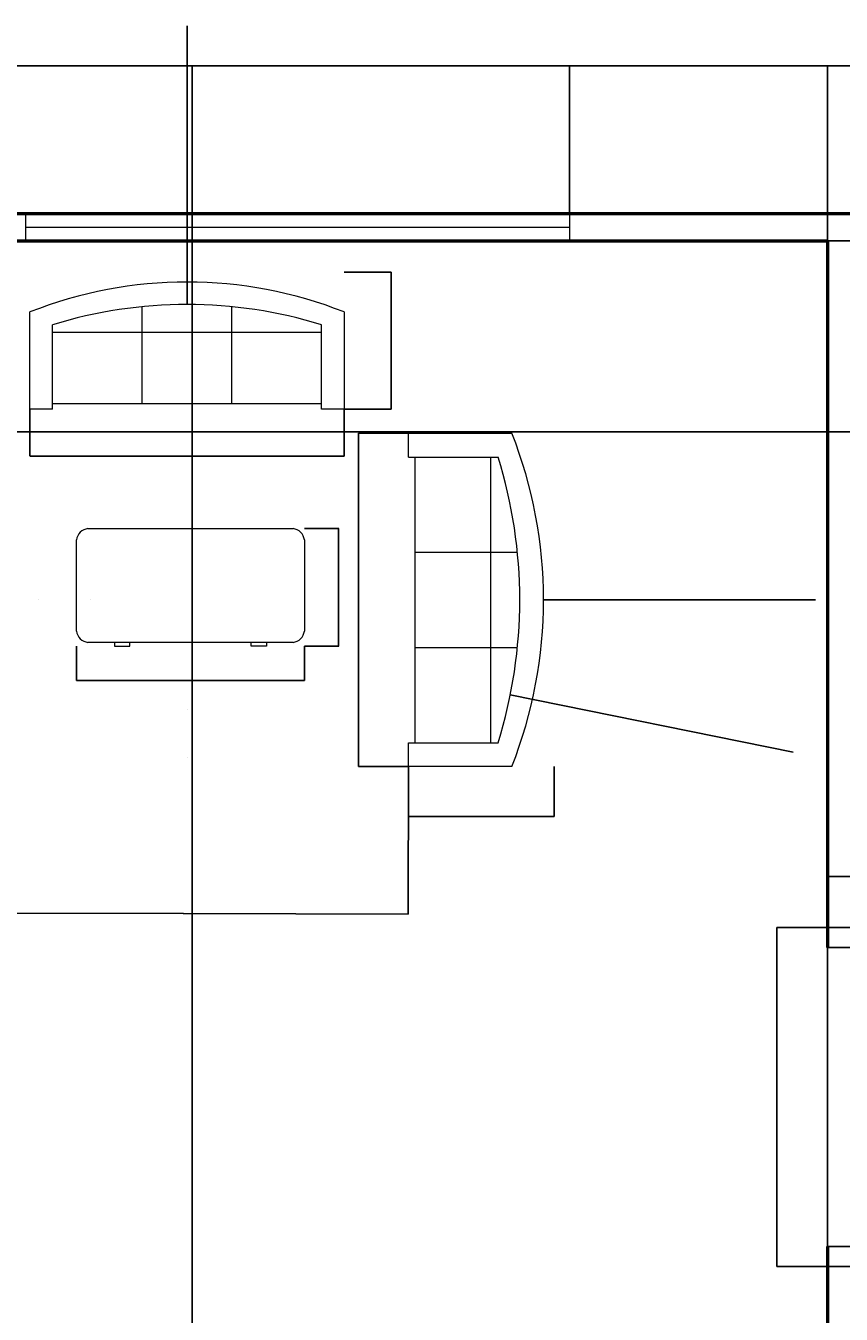
# Model space of a CAD drawing. Units: millimetres. Extents: x 1584 to 12772, y -932 to 10602.
# Tile 4 of 4: x 6178 to 9178, y 5860 to 10602. Entities that reach past the tile are written whole.
import ezdxf

# ---------------------------------------------------------------- set-up
doc = ezdxf.new("R2010")
doc.units = ezdxf.units.MM
for name, color, linetype, lineweight in [('A-ANNO-DIMS', 2, 'Continuous', 18), ('A-DOOR', 3, 'Continuous', 25), ('A-FURN', 8, 'Continuous', 18), ('A-GLAZ', 4, 'Continuous', 18), ('A-WALL', 7, 'Continuous', 50)]:
    doc.layers.add(name, color=color, linetype=linetype, lineweight=lineweight)
doc.styles.get("Standard").update_dxf_attribs({"font": 'arial.ttf'})
doc.dimstyles.get("Standard").update_dxf_attribs({"dimtxt": 0.18, "dimasz": 0.18, "dimexe": 0.18, "dimexo": 0.0625, "dimgap": 0.09, "dimtad": 0, "dimtih": 1, "dimtoh": 1, "dimdec": 4, "dimzin": 0, "dimdsep": 46, "dimtxsty": 'Standard', "dimcen": 0.09, "dimadec": 0, "dimazin": 0, "dimtfac": 1, "dimtdec": 4, "dimtofl": 0, "dimtmove": 0, "dimatfit": 3, "dimfxl": 1, "dimtolj": 1, "dimtzin": 0, "dimarcsym": 0})

# ---------------------------------------------------------------- blocks, each defined once
blk = doc.blocks.new('Sofa - Roundback 7 ft.')
for p, q in [((-12.00002, -32.44210000000393), (-12.00003, -6.597100000003898)), ((11.99996999999999, -32.44210000000393), (11.99997999999999, -6.597100000003898)), ((-36.000027, -34.00000000000395), (-36.000027, -11.46960000000396)), ((35.99997999999999, -34.00000000000395), (35.99997999999999, -11.46960000000396)), ((-35.999844, -13.38190000000397), (35.99979999999999, -13.38190000000397)), ((-36.000027, -32.44210000000393), (35.99997999999999, -32.44210000000393))]:
    blk.add_line(p, q)
for points in [[(-36.000027, -34.00000000000395), (-42.000027, -34.00000000000395), (-42.000027, -8.000000000003944)], [(41.99997999999999, -8.000000000003944), (41.99997999999999, -34.00000000000395), (35.99997999999999, -34.00000000000395)]]:
    blk.add_lwpolyline(points)
for centre, radius, start, end in [((0, -114.2500000000039), 114.2500000000039, 68.43141000000072, 111.5686000000006), ((-1.00000000032e-05, -127.1968000000039), 121.1967999999973, 72.72032999999948, 107.2797000000005)]:
    blk.add_arc(centre, radius, start, end)
blk = doc.blocks.new('Desk - 30 x 60 in.')
for p, q in [((-26.999995, 0), (26.999995, 0)), ((-29.999995, -27), (-29.999995, -3)), ((29.999995, -3), (29.999995, -27)), ((26.999995, -30), (-26.999995, -30)), ((-20.000005, -30), (-20.000005, -31)), ((-16.000005, -31), (-16.000005, -30)), ((15.999995, -31), (15.999995, -30)), ((19.999995, -30), (19.999995, -31)), ((-20.000005, -31), (-16.000005, -31)), ((19.999995, -31), (15.999995, -31))]:
    blk.add_line(p, q)
for centre, radius, start, end in [((-26.499995, -3.5), 3.535534000004229, 98.1300999999916, 171.8698999999352), ((26.499995, -3.5), 3.535533999997753, 8.130102000022115, 81.8698999999439), ((-26.499995, -26.5), 3.535534000000845, 188.1301000000653, 261.8699000000085), ((26.499995, -26.5), 3.535534000004826, 278.1301000000561, 351.8698999999439)]:
    blk.add_arc(centre, radius, start, end)
blk = doc.blocks.new('DOOR-SINGLE-1000')
for p, q in [((1000.000230036349, 1174.20008536707), (1000.000230036349, 1248.400085367071)), ((1000.000230036349, 1248.400085367071), (1100.000230036349, 1248.400085367071)), ((1100.000230036349, 1248.400085367071), (1100.000230036349, 1174.20008536707)), ((1000.000230036349, 1174.20008536707), (0.0002300363494214, 1174.20008536707)), ((0.0002300363494214, 1174.20008536707), (0.0002300363494214, 1074.200085367071)), ((1000.000230036349, 1074.200085367071), (1000.000230036349, 1174.20008536707)), ((1100.000230036349, 1174.20008536707), (1000.000230036349, 1174.20008536707)), ((0.0002300363494214, 1074.200085367071), (1000.000230036349, 1074.200085367071)), ((1000.000230036349, 8.53670690049e-05), (1000.000230036349, 74.20008536706973)), ((1000.000230036349, 74.20008536706973), (1100.000230036349, 74.20008536706973)), ((1100.000230036349, 74.20008536706973), (1100.000230036349, 8.53670690049e-05)), ((1100.000230036349, 8.53670690049e-05), (1000.000230036349, 8.53670690049e-05))]:
    blk.add_line(p, q)
blk.add_arc((1000.000230036349, 1074.200085367071), 1000.000000000001, 180, 270)
blk = doc.blocks.new('WIN-2000')
for p, q in [((-0.0004293290949136, 99.99960647437545), (1999.999570670905, 99.99960647437545)), ((-0.0004293290949136, -0.0003935256245313), (-0.0004293290949136, 99.99960647437545)), ((1999.999570670905, 99.99960647437545), (1999.999570670905, -0.0003935256245313)), ((-0.0004293290949136, 49.99960647437365), (1999.999570670905, 49.99960647437183)), ((1999.999570670905, -0.0003935256245313), (-0.0004293290949136, -0.0003935256245313))]:
    blk.add_line(p, q)
blk = doc.blocks.new('*D12')
at = {"layer": 'A-ANNO-DIMS', "color": 0, "lineweight": -2, "transparency": 16777216}
for p, q in [((9127.770730036345, 7283.820415011046), (8940.393230036349, 7283.820415011046)), ((8940.573230036349, 7283.640415011046), (8940.573230036349, 6659.803545979666)), ((8940.573230036349, 6035.600415011042), (8940.573230036349, 6659.437284042422)), ((9127.770730036345, 6035.420415011042), (8940.393230036349, 6035.420415011042))]:
    blk.add_line(p, q, dxfattribs=at)
at = {"layer": 'A-ANNO-DIMS', "color": 0, "transparency": 16777216}
for points in [[(8940.543230036348, 7283.640415011046), (8940.60323003635, 7283.640415011046), (8940.573230036349, 7283.820415011046)], [(8940.543230036348, 6035.600415011042), (8940.60323003635, 6035.600415011042), (8940.573230036349, 6035.420415011042)]]:
    blk.add_solid(points, dxfattribs=at)
at = {"layer": 'Defpoints', "color": 0, "transparency": 16777216}
for p in [(9127.833230036345, 7283.820415011046), (8940.573230036349, 6035.420415011042), (9127.833230036345, 6035.420415011042)]:
    blk.add_point(p, dxfattribs=at)
at = {"layer": 'A-ANNO-DIMS', "color": 0, "transparency": 16777216, "insert": (8940.573230036349, 6659.62041501104), "char_height": 0.18, "attachment_point": 5}
blk.add_mtext('\\A1;INTERNAL DOOR 1248 TYP.', dxfattribs=at)
blk = doc.blocks.new('*D13')
at = {"layer": 'A-ANNO-DIMS', "color": 0, "lineweight": -2, "transparency": 16777216}
for p, q in [((9127.833230036342, 7283.882915011043), (9127.833230036342, 7471.260415011044)), ((9128.013230036344, 7471.080415011043), (9677.173762096369, 7471.080415011043)), ((10227.65323003634, 7471.080415011043), (9678.492697976317, 7471.080415011043)), ((10227.83323003634, 7283.882915011043), (10227.83323003634, 7471.260415011044))]:
    blk.add_line(p, q, dxfattribs=at)
at = {"layer": 'A-ANNO-DIMS', "color": 0, "transparency": 16777216}
for points in [[(9128.013230036344, 7471.110415011043), (9128.013230036344, 7471.050415011044), (9127.833230036342, 7471.080415011043)], [(10227.65323003634, 7471.110415011043), (10227.65323003634, 7471.050415011044), (10227.83323003634, 7471.080415011043)]]:
    blk.add_solid(points, dxfattribs=at)
at = {"layer": 'Defpoints', "color": 0, "transparency": 16777216}
for p in [(9127.833230036342, 7471.080415011043), (9127.833230036342, 7283.820415011042), (10227.83323003634, 7283.820415011042)]:
    blk.add_point(p, dxfattribs=at)
at = {"layer": 'A-ANNO-DIMS', "color": 0, "transparency": 16777216, "insert": (9677.833230036342, 7471.080415011043), "char_height": 0.18, "attachment_point": 5}
blk.add_mtext('\\A1;1100 TYP.', dxfattribs=at)
blk = doc.blocks.new('*D16')
at = {"layer": 'A-ANNO-DIMS', "color": 0, "lineweight": -2, "transparency": 16777216}
for p, q in [((7586.315416002381, 9102.27341029342), (7402.236101158712, 9102.27341029342)), ((7402.416101158713, 9102.093410293419), (7402.416101158713, 8489.250491783136)), ((7402.416101158713, 7876.041311335602), (7402.416101158713, 8488.88422984589)), ((7586.315416002381, 7875.861311335602), (7402.236101158712, 7875.861311335602))]:
    blk.add_line(p, q, dxfattribs=at)
at = {"layer": 'A-ANNO-DIMS', "color": 0, "transparency": 16777216}
for points in [[(7402.386101158713, 9102.093410293419), (7402.446101158712, 9102.093410293419), (7402.416101158713, 9102.27341029342)], [(7402.386101158713, 7876.041311335602), (7402.446101158712, 7876.041311335602), (7402.416101158713, 7875.861311335602)]]:
    blk.add_solid(points, dxfattribs=at)
at = {"layer": 'Defpoints', "color": 0, "transparency": 16777216}
for p in [(7586.377916002381, 9102.27341029342), (7402.416101158713, 7875.861311335602), (7586.377916002381, 7875.861311335602)]:
    blk.add_point(p, dxfattribs=at)
at = {"layer": 'A-ANNO-DIMS', "color": 0, "transparency": 16777216, "insert": (7402.416101158713, 8489.067360814506), "char_height": 0.18, "attachment_point": 5}
blk.add_mtext('\\A1;SOFA 1226 TYP.', dxfattribs=at)
blk = doc.blocks.new('*D17')
at = {"layer": 'A-ANNO-DIMS', "color": 0, "lineweight": -2, "transparency": 16777216}
for p, q in [((7586.377916002378, 7875.798811335599), (7586.377916002378, 7691.719496491926)), ((8121.716442842506, 7875.798811335599), (8121.716442842506, 7691.719496491926)), ((7586.557916002378, 7691.899496491926), (7853.449164415621, 7691.899496491926)), ((8121.536442842506, 7691.899496491926), (7854.645194429264, 7691.899496491926))]:
    blk.add_line(p, q, dxfattribs=at)
at = {"layer": 'A-ANNO-DIMS', "color": 0, "transparency": 16777216}
for points in [[(7586.557916002378, 7691.929496491926), (7586.557916002378, 7691.869496491925), (7586.377916002378, 7691.899496491926)], [(8121.536442842506, 7691.929496491926), (8121.536442842506, 7691.869496491925), (8121.716442842506, 7691.899496491926)]]:
    blk.add_solid(points, dxfattribs=at)
at = {"layer": 'Defpoints', "color": 0, "transparency": 16777216}
for p in [(7586.377916002378, 7875.861311335599), (8121.716442842506, 7875.861311335599), (8121.716442842506, 7691.899496491926)]:
    blk.add_point(p, dxfattribs=at)
at = {"layer": 'A-ANNO-DIMS', "color": 0, "transparency": 16777216, "insert": (7854.047179422443, 7691.899496491926), "char_height": 0.18, "attachment_point": 5}
blk.add_mtext('\\A1;535 TYP.', dxfattribs=at)
blk = doc.blocks.new('*D18')
at = {"layer": 'A-ANNO-DIMS', "color": 0, "lineweight": -2, "transparency": 16777216}
for p, q in [((6193.307512875763, 9190.657173150928), (6193.307512875763, 9017.202769135929)), ((7348.886872975739, 9190.657173150928), (7348.886872975739, 9017.202769135929)), ((6193.487512875763, 9017.38276913593), (6770.361660865724, 9017.38276913593)), ((7348.706872975739, 9017.38276913593), (6771.832724985777, 9017.38276913593))]:
    blk.add_line(p, q, dxfattribs=at)
at = {"layer": 'A-ANNO-DIMS', "color": 0, "transparency": 16777216}
for points in [[(6193.487512875763, 9017.41276913593), (6193.487512875763, 9017.352769135929), (6193.307512875763, 9017.38276913593)], [(7348.706872975739, 9017.41276913593), (7348.706872975739, 9017.352769135929), (7348.886872975739, 9017.38276913593)]]:
    blk.add_solid(points, dxfattribs=at)
at = {"layer": 'Defpoints', "color": 0, "transparency": 16777216}
for p in [(6193.307512875763, 9190.719673150928), (7348.886872975739, 9190.719673150928), (7348.886872975739, 9017.38276913593)]:
    blk.add_point(p, dxfattribs=at)
at = {"layer": 'A-ANNO-DIMS', "color": 0, "transparency": 16777216, "insert": (6771.097192925751, 9017.38276913593), "char_height": 0.18, "attachment_point": 5}
blk.add_mtext('\\A1;SOFA 1156', dxfattribs=at)
blk = doc.blocks.new('*D19')
at = {"layer": 'A-ANNO-DIMS', "color": 0, "lineweight": -2, "transparency": 16777216}
for p, q in [((7348.949372975742, 9695.139152385094), (7522.403776990744, 9695.139152385094)), ((7522.223776990744, 9694.959152385096), (7522.223776990744, 9443.111315905802)), ((7522.223776990744, 9190.899673150932), (7522.223776990744, 9442.747509630224)), ((7348.949372975742, 9190.71967315093), (7522.403776990744, 9190.71967315093))]:
    blk.add_line(p, q, dxfattribs=at)
at = {"layer": 'A-ANNO-DIMS', "color": 0, "transparency": 16777216}
for points in [[(7522.193776990744, 9694.959152385096), (7522.253776990743, 9694.959152385096), (7522.223776990744, 9695.139152385094)], [(7522.193776990744, 9190.899673150932), (7522.253776990743, 9190.899673150932), (7522.223776990744, 9190.71967315093)]]:
    blk.add_solid(points, dxfattribs=at)
at = {"layer": 'Defpoints', "color": 0, "transparency": 16777216}
for p in [(7348.886872975743, 9695.139152385094), (7522.223776990744, 9695.139152385094), (7348.886872975743, 9190.71967315093)]:
    blk.add_point(p, dxfattribs=at)
at = {"layer": 'A-ANNO-DIMS', "color": 0, "transparency": 16777216, "insert": (7522.223776990744, 9442.92941276801), "char_height": 0.18, "attachment_point": 5}
blk.add_mtext('\\A1;504', dxfattribs=at)
blk = doc.blocks.new('*D30')
at = {"layer": 'A-ANNO-DIMS', "color": 0, "lineweight": -2, "transparency": 16777216}
for p, q in [((6364.313560520749, 8318.107093990797), (6364.313560520749, 8192.188321129659)), ((7202.988712928337, 8318.107093990797), (7202.988712928337, 8192.188321129659)), ((6364.49356052075, 8192.36832112966), (6782.989274514448, 8192.36832112966)), ((7202.808712928336, 8192.36832112966), (6784.312998934639, 8192.36832112966))]:
    blk.add_line(p, q, dxfattribs=at)
at = {"layer": 'A-ANNO-DIMS', "color": 0, "transparency": 16777216}
for points in [[(6364.49356052075, 8192.39832112966), (6364.49356052075, 8192.338321129659), (6364.313560520749, 8192.36832112966)], [(7202.808712928336, 8192.39832112966), (7202.808712928336, 8192.338321129659), (7202.988712928337, 8192.36832112966)]]:
    blk.add_solid(points, dxfattribs=at)
at = {"layer": 'Defpoints', "color": 0, "transparency": 16777216}
for p in [(6364.313560520749, 8318.169593990797), (7202.988712928337, 8318.169593990797), (7202.988712928337, 8192.36832112966)]:
    blk.add_point(p, dxfattribs=at)
at = {"layer": 'A-ANNO-DIMS', "color": 0, "transparency": 16777216, "insert": (6783.651136724543, 8192.36832112966), "char_height": 0.18, "attachment_point": 5}
blk.add_mtext('\\A1;DESK 839', dxfattribs=at)
blk = doc.blocks.new('*D31')
at = {"layer": 'A-ANNO-DIMS', "color": 0, "lineweight": -2, "transparency": 16777216}
for p, q in [((7203.05121292834, 8751.48516156769), (7328.969985789481, 8751.48516156769)), ((7328.789985789481, 8751.30516156769), (7328.789985789481, 8535.009342308576)), ((7328.789985789481, 8318.3495939908), (7328.789985789481, 8534.645413249915)), ((7203.05121292834, 8318.1695939908), (7328.969985789481, 8318.1695939908))]:
    blk.add_line(p, q, dxfattribs=at)
at = {"layer": 'A-ANNO-DIMS', "color": 0, "transparency": 16777216}
for points in [[(7328.759985789481, 8751.30516156769), (7328.819985789481, 8751.30516156769), (7328.789985789481, 8751.48516156769)], [(7328.759985789481, 8318.3495939908), (7328.819985789481, 8318.3495939908), (7328.789985789481, 8318.1695939908)]]:
    blk.add_solid(points, dxfattribs=at)
at = {"layer": 'Defpoints', "color": 0, "transparency": 16777216}
for p in [(7202.988712928339, 8751.48516156769), (7328.789985789481, 8751.48516156769), (7202.988712928339, 8318.1695939908)]:
    blk.add_point(p, dxfattribs=at)
at = {"layer": 'A-ANNO-DIMS', "color": 0, "transparency": 16777216, "insert": (7328.789985789481, 8534.827377779242), "char_height": 0.18, "attachment_point": 5}
blk.add_mtext('\\A1;433', dxfattribs=at)
blk = doc.blocks.new('*D37')
at = {"layer": 'A-ANNO-DIMS', "color": 0, "lineweight": -2, "transparency": 16777216}
for p, q in [((12227.89573, 9910.180606000004), (12771.71323000001, 9910.180606000005)), ((12771.53323000001, 9910.000606000005), (12771.53323000001, 4761.453150137792)), ((12771.53323000001, -387.4581119999995), (12771.53323000001, 4761.089343862212)), ((8227.895730000006, -387.6381120000002), (12771.71323000001, -387.6381119999995))]:
    blk.add_line(p, q, dxfattribs=at)
at = {"layer": 'A-ANNO-DIMS', "color": 0, "transparency": 16777216}
for points in [[(12771.50323000001, 9910.000606000005), (12771.56323000001, 9910.000606000005), (12771.53323000001, 9910.180606000005)], [(12771.50323000001, -387.4581119999995), (12771.56323000001, -387.4581119999995), (12771.53323000001, -387.6381119999995)]]:
    blk.add_solid(points, dxfattribs=at)
at = {"layer": 'Defpoints', "color": 0, "transparency": 16777216}
for p in [(12227.83323, 9910.180606000004), (12771.53323000001, 9910.180606000005), (8227.833230000006, -387.6381120000002)]:
    blk.add_point(p, dxfattribs=at)
at = {"layer": 'A-ANNO-DIMS', "color": 0, "transparency": 16777216, "insert": (12771.53323000001, 4761.271246999998), "char_height": 0.18, "attachment_point": 5}
blk.add_mtext('\\A1;10298', dxfattribs=at)
blk = doc.blocks.new('*D44')
at = {"layer": 'A-ANNO-DIMS', "color": 0, "lineweight": -2, "transparency": 16777216}
for p, q in [((5227.83323, 312.424388), (5227.833230000001, 10454.060606)), ((5228.013230000001, 10453.880606), (7177.474826180082, 10453.880606)), ((9127.65323, 10453.880606), (7178.191633819918, 10453.880606)), ((9127.83323, 312.424388), (9127.83323, 10454.060606))]:
    blk.add_line(p, q, dxfattribs=at)
at = {"layer": 'A-ANNO-DIMS', "color": 0, "transparency": 16777216}
for points in [[(5228.013230000001, 10453.910606), (5228.013230000001, 10453.850606), (5227.833230000001, 10453.880606)], [(9127.65323, 10453.910606), (9127.65323, 10453.850606), (9127.83323, 10453.880606)]]:
    blk.add_solid(points, dxfattribs=at)
at = {"layer": 'Defpoints', "color": 0, "transparency": 16777216}
for p in [(9127.83323, 10453.880606), (5227.83323, 312.361888), (9127.83323, 312.361888)]:
    blk.add_point(p, dxfattribs=at)
at = {"layer": 'A-ANNO-DIMS', "color": 0, "transparency": 16777216, "insert": (7177.83323, 10453.880606), "char_height": 0.18, "attachment_point": 5}
blk.add_mtext('\\A1;3900', dxfattribs=at)
blk = doc.blocks.new('*D53')
at = {"layer": 'A-ANNO-DIMS', "color": 0, "lineweight": -2, "transparency": 16777216}
for p, q in [((8177.781093, 9910.243106000002), (8177.781093, 10454.060606)), ((8177.961093, 10453.880606), (8931.027043459755, 10453.880606)), ((9685.002571, 10453.880606), (8931.936620540248, 10453.880606)), ((9685.182571, 9910.243106000002), (9685.182571, 10454.060606))]:
    blk.add_line(p, q, dxfattribs=at)
at = {"layer": 'A-ANNO-DIMS', "color": 0, "transparency": 16777216}
for points in [[(8177.961093, 10453.910606), (8177.961093, 10453.850606), (8177.781093, 10453.880606)], [(9685.002571, 10453.910606), (9685.002571, 10453.850606), (9685.182571, 10453.880606)]]:
    blk.add_solid(points, dxfattribs=at)
at = {"layer": 'Defpoints', "color": 0, "transparency": 16777216}
for p in [(9685.182571, 10453.880606), (8177.781093, 9910.180606), (9685.182571, 9910.180606)]:
    blk.add_point(p, dxfattribs=at)
at = {"layer": 'A-ANNO-DIMS', "color": 0, "transparency": 16777216, "insert": (8931.481832000001, 10453.880606), "char_height": 0.18, "attachment_point": 5}
blk.add_mtext('\\A1;1507.4', dxfattribs=at)
blk = doc.blocks.new('*D72')
at = {"layer": 'A-ANNO-DIMS', "color": 0, "lineweight": -2, "transparency": 16777216}
for p, q in [((5227.83323, 4478.976585), (5227.83323, 10454.060606)), ((5228.013230000001, 10453.880606), (6008.25544143588, 10453.880606)), ((6789.408335, 10453.880606), (6009.166123564121, 10453.880606)), ((6789.588335000001, 4491.747446999999), (6789.588335000001, 10454.060606))]:
    blk.add_line(p, q, dxfattribs=at)
at = {"layer": 'A-ANNO-DIMS', "color": 0, "transparency": 16777216}
for points in [[(5228.013230000001, 10453.910606), (5228.013230000001, 10453.850606), (5227.83323, 10453.880606)], [(6789.408335, 10453.910606), (6789.408335, 10453.850606), (6789.588335000001, 10453.880606)]]:
    blk.add_solid(points, dxfattribs=at)
at = {"layer": 'Defpoints', "color": 0, "transparency": 16777216}
for p in [(6789.588335000001, 10453.880606), (5227.83323, 4478.914085), (6789.588335000001, 4491.684946999999)]:
    blk.add_point(p, dxfattribs=at)
at = {"layer": 'A-ANNO-DIMS', "color": 0, "transparency": 16777216, "insert": (6008.7107825, 10453.880606), "char_height": 0.18, "attachment_point": 5}
blk.add_mtext('\\A1;1561.8', dxfattribs=at)
blk = doc.blocks.new('*D74')
at = {"layer": 'A-ANNO-DIMS', "color": 0, "lineweight": -2, "transparency": 16777216}
for p, q in [((5930.629051045201, 7880.354388236549), (5929.1328585744, 7336.538946787445)), ((7586.377744045201, 7875.798948236547), (7584.881551573826, 7331.9835065789)), ((5929.313353122965, 7336.718450876363), (6756.552359239816, 7334.442478775962)), ((7584.702047484907, 7332.164001127465), (6757.463041368056, 7334.439973227866))]:
    blk.add_line(p, q, dxfattribs=at)
at = {"layer": 'A-ANNO-DIMS', "color": 0, "transparency": 16777216}
for points in [[(5929.313435661269, 7336.748450762819), (5929.31327058466, 7336.688450989905), (5929.133353804224, 7336.718946106187)], [(7584.702130023211, 7332.194001013923), (7584.701964946603, 7332.134001241009), (7584.882046803651, 7332.163505897641)]]:
    blk.add_solid(points, dxfattribs=at)
at = {"layer": 'Defpoints', "color": 0, "transparency": 16777216}
for p in [(5930.629223000001, 7880.416888), (7586.377916000002, 7875.861447999999), (5929.133353804224, 7336.718946106187)]:
    blk.add_point(p, dxfattribs=at)
at = {"layer": 'A-ANNO-DIMS', "color": 0, "transparency": 16777216, "insert": (6757.007700303936, 7334.441226001914), "char_height": 0.18, "attachment_point": 5}
blk.add_mtext('\\A1;1655.8', dxfattribs=at)
blk = doc.blocks.new('*D75')
at = {"layer": 'A-ANNO-DIMS', "color": 0, "lineweight": -2, "transparency": 16777216}
for p, q in [((5227.895730000002, 9810.180606000004), (12771.71323000001, 9810.180606000005)), ((12771.53323000001, 9810.000606000007), (12771.53323000001, 9458.68676102934)), ((12771.53323000001, 9107.008987000005), (12771.53323000001, 9458.322831970676)), ((5551.087991000002, 9106.828987000004), (12771.71323000001, 9106.828987000004))]:
    blk.add_line(p, q, dxfattribs=at)
at = {"layer": 'A-ANNO-DIMS', "color": 0, "transparency": 16777216}
for points in [[(12771.50323000001, 9810.000606000007), (12771.56323000001, 9810.000606000007), (12771.53323000001, 9810.180606000005)], [(12771.50323000001, 9107.008987000005), (12771.56323000001, 9107.008987000005), (12771.53323000001, 9106.828987000004)]]:
    blk.add_solid(points, dxfattribs=at)
at = {"layer": 'Defpoints', "color": 0, "transparency": 16777216}
for p in [(5227.833230000002, 9810.180606000004), (5551.025491000002, 9106.828987000004), (12771.53323000001, 9106.828987000004)]:
    blk.add_point(p, dxfattribs=at)
at = {"layer": 'A-ANNO-DIMS', "color": 0, "transparency": 16777216, "insert": (12771.53323000001, 9458.504796500001), "char_height": 0.18, "attachment_point": 5}
blk.add_mtext('\\A1;703.4', dxfattribs=at)
blk = doc.blocks.new('*D81')
at = {"layer": 'A-ANNO-DIMS', "color": 0, "lineweight": -2, "transparency": 16777216}
for p, q in [((6225.601477, 8489.067231999998), (6225.781477, 8489.067232)), ((6225.691477, 8488.977231999996), (6225.691476999999, 8489.157231999998)), ((9000.918127772267, 7928.957033686327), (7960.384576324607, 8138.96274752278))]:
    blk.add_line(p, q, dxfattribs=at)
at = {"layer": 'A-ANNO-DIMS', "color": 0, "transparency": 16777216}
blk.add_solid([(7960.390511404144, 8138.992154576882), (7960.37864124507, 8138.93334046868), (7960.208134000001, 8138.998358)], dxfattribs=at)
at = {"layer": 'Defpoints', "color": 0, "transparency": 16777216}
for p in [(6225.691477, 8489.067231999998), (7960.208134000001, 8138.998358)]:
    blk.add_point(p, dxfattribs=at)
at = {"layer": 'A-ANNO-DIMS', "color": 0, "transparency": 16777216, "insert": (9001.66348247895, 7928.957033686327), "char_height": 0.18, "attachment_point": 5}
blk.add_mtext('\\A1;2X R1769.5', dxfattribs=at)
blk = doc.blocks.new('*D82')
at = {"layer": 'A-ANNO-DIMS', "color": 0, "lineweight": -2, "transparency": 16777216}
for p, q in [((6414.626585000002, 8489.067086000003), (6414.806585000002, 8489.067086000003)), ((6414.716585000002, 8488.977086000003), (6414.716585000002, 8489.157086000005)), ((9083.622394599997, 8489.0669484), (8082.962715999999, 8489.06699999072))]:
    blk.add_line(p, q, dxfattribs=at)
at = {"layer": 'A-ANNO-DIMS', "color": 0, "transparency": 16777216}
blk.add_solid([(8082.962716001544, 8489.096999990721), (8082.962715998453, 8489.03699999072), (8082.782715999998, 8489.067000000003)], dxfattribs=at)
at = {"layer": 'Defpoints', "color": 0, "transparency": 16777216}
for p in [(6414.716585, 8489.067086000003), (8082.782715999998, 8489.067000000003)]:
    blk.add_point(p, dxfattribs=at)
at = {"layer": 'A-ANNO-DIMS', "color": 0, "transparency": 16777216, "insert": (9084.262401421278, 8489.0669484), "char_height": 0.18, "attachment_point": 5}
blk.add_mtext('\\A1;2X R1668', dxfattribs=at)
blk = doc.blocks.new('*D83')
at = {"layer": 'A-ANNO-DIMS', "color": 0, "lineweight": -2, "transparency": 16777216}
for p, q in [((6771.277000000006, 10576.2876702), (6771.097000000006, 10576.2876702)), ((6771.097000000006, 10576.2876702), (6771.097000000008, 9576.092718000007)), ((6771.007314000006, 7908.621131000007), (6771.187314000006, 7908.621131000007)), ((6771.097314000006, 7908.531131000007), (6771.097314000006, 7908.711131000007))]:
    blk.add_line(p, q, dxfattribs=at)
at = {"layer": 'A-ANNO-DIMS', "color": 0, "transparency": 16777216}
blk.add_solid([(6771.067000000008, 9576.092718000007), (6771.127000000007, 9576.092718000007), (6771.097000000008, 9575.912718000007)], dxfattribs=at)
at = {"layer": 'Defpoints', "color": 0, "transparency": 16777216}
for p in [(6771.097000000008, 9575.912718000007), (6771.097314000006, 7908.621131000007)]:
    blk.add_point(p, dxfattribs=at)
at = {"layer": 'A-ANNO-DIMS', "color": 0, "transparency": 16777216, "insert": (6771.826761255123, 10576.2876702), "char_height": 0.18, "attachment_point": 5}
blk.add_mtext('\\A1;R1667.3', dxfattribs=at)
blk = doc.blocks.new('*D84')
at = {"layer": 'A-ANNO-DIMS', "color": 0, "lineweight": -2, "transparency": 16777216}
for p, q in [((6771.277000000006, 10601.4892008), (6771.097000000006, 10601.4892008)), ((6771.097000000006, 10601.4892008), (6771.097000000008, 9658.634085000009)), ((6771.007452000008, 8086.728892000008), (6771.187452000008, 8086.728892000008)), ((6771.097452000008, 8086.638892000008), (6771.097452000008, 8086.818892000009))]:
    blk.add_line(p, q, dxfattribs=at)
at = {"layer": 'A-ANNO-DIMS', "color": 0, "transparency": 16777216}
blk.add_solid([(6771.067000000008, 9658.634085000009), (6771.127000000007, 9658.634085000009), (6771.097000000008, 9658.454085000007)], dxfattribs=at)
at = {"layer": 'Defpoints', "color": 0, "transparency": 16777216}
for p in [(6771.097000000008, 9658.454085000007), (6771.097452000008, 8086.728892000008)]:
    blk.add_point(p, dxfattribs=at)
at = {"layer": 'A-ANNO-DIMS', "color": 0, "transparency": 16777216, "insert": (6771.826761255123, 10601.4892008), "char_height": 0.18, "attachment_point": 5}
blk.add_mtext('\\A1;R1571.7', dxfattribs=at)

msp = doc.modelspace()

# ---------------------------------------------------------------- linework, layer by layer
at = {"layer": 'A-WALL'}
for p, q in [((2127.833230036349, 9910.180606474376), (12227.83323003635, 9910.180606474376)), ((5227.833230036349, 9810.18060647438), (9127.833230036353, 9810.18060647438)), ((9127.83323003635, 9810.18060647438), (9127.83323003635, 7209.620415011039)), ((9127.833230036349, 6109.620415011038), (9127.833230036349, 5910.180606474376)), ((9127.83323003635, 5910.180606474376), (9127.833230036349, 5810.180606474376))]:
    msp.add_line(p, q, dxfattribs=at)

# ---------------------------------------------------------------- block references
at = {"layer": 'A-DOOR', "rotation": 180}
msp.add_blockref('DOOR-SINGLE-1000', (10227.83346007269, 7283.820500378111), dxfattribs=at)
at = {"layer": 'A-FURN'}
for name, p, xscale, yscale, zscale in [('Sofa - Roundback 7 ft.', (6771.097451798087, 9658.454084925503), 13.75689446395651, 13.75689446395651, 13.75689446395651), ('Desk - 30 x 60 in.', (6783.651136724538, 8751.485159978816), 13.9779214834845, 13.9779214834845, 13.9779214834845)]:
    msp.add_blockref(name, p, dxfattribs=dict(at, xscale=xscale, yscale=yscale, zscale=zscale))
at = {"layer": 'A-FURN', "xscale": 14.60014119084165, "yscale": 14.60014119084165, "zscale": 14.60014119084165, "rotation": 270}
msp.add_blockref('Sofa - Roundback 7 ft.', (8082.782716491051, 8489.067086074256), dxfattribs=at)
at = {"layer": 'A-GLAZ'}
msp.add_blockref('WIN-2000', (6177.781522690212, 9810.181), dxfattribs=at)

# ---------------------------------------------------------------- dimensions: what is measured, and where the dimension line sits
at = {"layer": 'A-ANNO-DIMS'}
for center, mpoint, picture, middle in [((6771.097314000006, 7908.621131000007), (6771.097000000008, 9575.912718000007), '*D83', (6771.826761255123, 10576.2876702)), ((6771.097452000008, 8086.728892000008), (6771.097000000008, 9658.454085000007), '*D84', (6771.826761255123, 10601.4892008))]:
    dim = msp.add_radius_dim(center=center, mpoint=mpoint, dimstyle='Standard', override={"dimdec": 1, "dimlfac": 1, "dimrnd": 0, "dimzin": 0, "dimdsep": 46, "dimlunit": 2}, dxfattribs=at)
    dim.commit()
    dim.dimension.update_dxf_attribs({"geometry": picture, "text_midpoint": middle, "dimtype": 164})
for base, p1, p2, override, picture, middle in [((9127.83323, 10453.880606), (5227.83323, 312.361888), (9127.83323, 312.361888), {"dimdec": 0, "dimlfac": 1, "dimrnd": 0, "dimzin": 0, "dimdsep": 46, "dimlunit": 2}, '*D44', (7177.83323, 10453.880606)), ((6789.588335000001, 10453.880606), (5227.83323, 4478.914085), (6789.588335000001, 4491.684946999999), {"dimdec": 1, "dimlfac": 1, "dimrnd": 0, "dimzin": 0, "dimdsep": 46, "dimlunit": 2}, '*D72', (6008.7107825, 10453.880606)), ((9685.182571, 10453.880606), (8177.781093, 9910.180606), (9685.182571, 9910.180606), {"dimdec": 1, "dimlfac": 1, "dimrnd": 0, "dimzin": 0, "dimdsep": 46, "dimlunit": 2}, '*D53', (8931.481832000001, 10453.880606))]:
    dim = msp.add_linear_dim(base=base, p1=p1, p2=p2, dimstyle='Standard', override=override, dxfattribs=at)
    dim.commit()
    dim.dimension.update_dxf_attribs({"geometry": picture, "text_midpoint": middle})
for base, p1, p2, angle, override, picture, middle in [((12771.53323000001, 9910.180606000005), (8227.833229999998, -387.638112), (12227.83323, 9910.180606), 90, {"dimdec": 0, "dimlfac": 1, "dimrnd": 0, "dimzin": 0, "dimdsep": 46, "dimlunit": 2}, '*D37', (12771.53323000001, 4761.271246999998)), ((12771.53323000001, 9106.828987000004), (5227.83323, 9810.180606000002), (5551.025491, 9106.828987), 90, {"dimdec": 1, "dimlfac": 1, "dimrnd": 0, "dimzin": 0, "dimdsep": 46, "dimlunit": 2}, '*D75', (12771.53323000001, 9458.504796500001)), ((7522.223776990744, 9695.139152385094), (7348.886872975739, 9190.719673150928), (7348.886872975739, 9695.139152385093), 90, {"dimdec": 0, "dimlfac": 1, "dimrnd": 0, "dimzin": 0, "dimdsep": 46, "dimlunit": 2}, '*D19', (7522.223776990744, 9442.92941276801)), ((7328.789985789481, 8751.48516156769), (7202.988712928337, 8318.169593990797), (7202.988712928337, 8751.485161567687), 90, {"dimdec": 0, "dimlfac": 1, "dimrnd": 0, "dimzin": 0, "dimdsep": 46, "dimlunit": 2}, '*D31', (7328.789985789481, 8534.827377779242)), ((5929.133353804224, 7336.718946106187), (7586.377916, 7875.861447999999), (5930.629223, 7880.416888), 179.8423632521602, {"dimdec": 1, "dimlfac": 1, "dimrnd": 0, "dimzin": 0, "dimdsep": 46, "dimlunit": 2}, '*D74', (6757.007700303936, 7334.441226001914))]:
    dim = msp.add_linear_dim(base=base, p1=p1, p2=p2, angle=angle, dimstyle='Standard', override=override, dxfattribs=at)
    dim.commit()
    dim.dimension.update_dxf_attribs({"geometry": picture, "text_midpoint": middle})
for base, p1, p2, text, picture, middle in [((7348.886872975739, 9017.38276913593), (6193.307512875763, 9190.719673150928), (7348.886872975739, 9190.719673150928), 'SOFA <>', '*D18', (6771.097192925751, 9017.38276913593)), ((7202.988712928337, 8192.36832112966), (6364.313560520749, 8318.169593990797), (7202.988712928337, 8318.169593990797), 'DESK <>', '*D30', (6783.651136724543, 8192.36832112966)), ((8121.716442842506, 7691.899496491926), (7586.377916002378, 7875.861311335599), (8121.716442842506, 7875.861311335599), '<> TYP.', '*D17', (7854.047179422443, 7691.899496491926))]:
    dim = msp.add_linear_dim(base=base, p1=p1, p2=p2, text=text, dimstyle='Standard', override={"dimdec": 0, "dimlfac": 1, "dimrnd": 0, "dimzin": 0, "dimdsep": 46, "dimlunit": 2}, dxfattribs=at)
    dim.commit()
    dim.dimension.update_dxf_attribs({"geometry": picture, "text_midpoint": middle})
for base, p1, p2, angle, text, picture, middle in [((7402.416101158713, 7875.861311335602), (7586.377916002378, 9102.273410293416), (7586.377916002378, 7875.861311335599), 270, 'SOFA <> TYP.', '*D16', (7402.416101158713, 8489.067360814506)), ((9127.833230036342, 7471.080415011043), (10227.83323003634, 7283.820415011042), (9127.833230036342, 7283.820415011042), 180, '<> TYP.', '*D13', (9677.833230036342, 7471.080415011043)), ((8940.573230036349, 6035.420415011042), (9127.833230036342, 7283.820415011042), (9127.833230036342, 6035.420415011041), 270, 'INTERNAL DOOR <> TYP.', '*D12', (8940.573230036349, 6659.62041501104))]:
    dim = msp.add_linear_dim(base=base, p1=p1, p2=p2, angle=angle, text=text, dimstyle='Standard', override={"dimdec": 0, "dimlfac": 1, "dimrnd": 0, "dimzin": 0, "dimdsep": 46, "dimlunit": 2}, dxfattribs=at)
    dim.commit()
    dim.dimension.update_dxf_attribs({"geometry": picture, "text_midpoint": middle})
for center, mpoint, override, picture, middle in [((6225.691477, 8489.067231999998), (7960.208134000001, 8138.998358), {"dimdec": 1, "dimlfac": 1, "dimrnd": 0, "dimzin": 0, "dimdsep": 46, "dimlunit": 2}, '*D81', (9000.918127772267, 7928.957033686327)), ((6414.716585, 8489.067086000003), (8082.782715999998, 8489.067000000003), {"dimdec": 0, "dimlfac": 1, "dimrnd": 0, "dimzin": 0, "dimdsep": 46, "dimlunit": 2}, '*D82', (9083.622394599997, 8489.0669484))]:
    dim = msp.add_radius_dim(center=center, mpoint=mpoint, text='2X <>', dimstyle='Standard', override=override, dxfattribs=at)
    dim.commit()
    dim.dimension.update_dxf_attribs({"geometry": picture, "text_midpoint": middle, "dimtype": 164})

doc.saveas('drawing.dxf')
